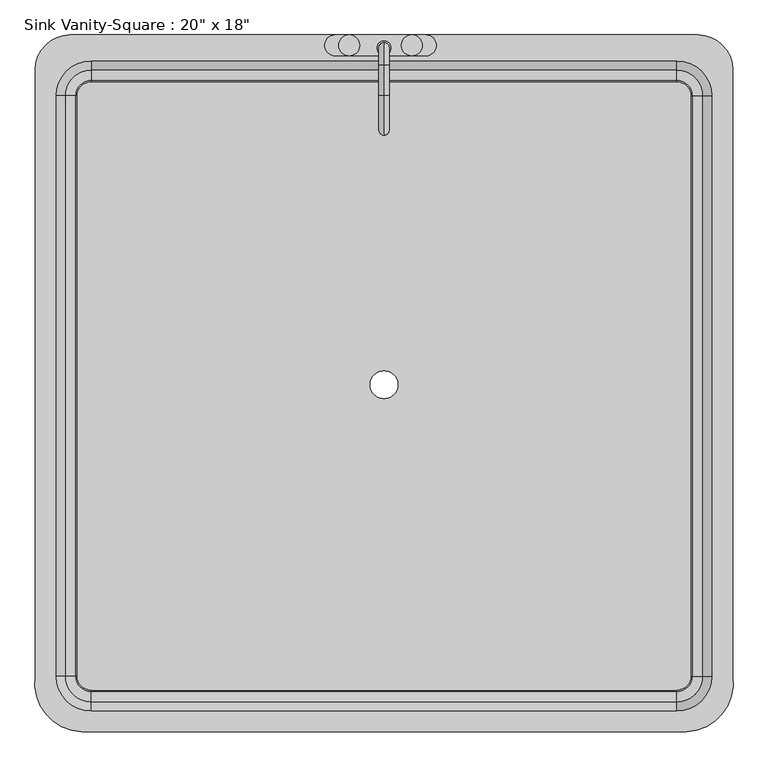
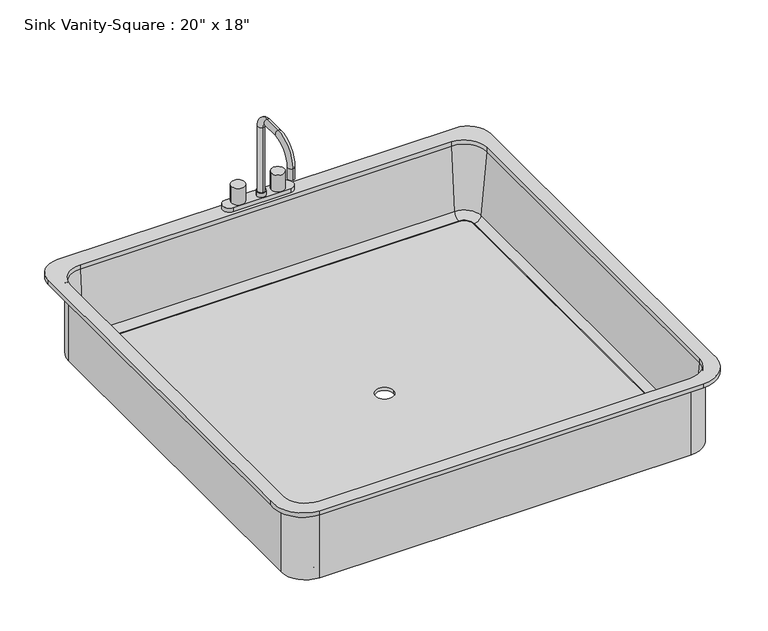
"""IFC4 building model written with IfcOpenShell, lengths in millimetres: flow terminal geometry."""

from ifc_helpers import new_model, si_unit, point, frame, frame_2d, origin, place, context, project, spatial, polyline, circle_curve, ellipse_curve, trimmed, segment, composite_curve, outline, extrude, source, transform, mapped, element, save
from ifc_brep_helpers import plane_surface, cylinder_surface, revolved_surface, advanced_brep


def flow_terminal_6a24c7e0(model_context):
    return source(origin(), model_context, "Body", "SolidModel", [
        extrude(outline(composite_curve([segment(trimmed(circle_curve(frame_2d((549.0892406, 475.4204011)), 25.4), [point((549.0892406, 500.8204011))], [point((574.4892406, 475.4204011))], False, "CARTESIAN"), True, "CONTINUOUS"), segment(polyline([(574.4892406, 475.4204011), (574.4892406, -581.8545989)]), True, "CONTINUOUS"), segment(trimmed(circle_curve(frame_2d((549.0892406, -581.8545989)), 25.4), [point((574.4892406, -581.8545989))], [point((549.0892406, -607.2545989))], False, "CARTESIAN"), True, "CONTINUOUS"), segment(polyline([(549.0892406, -607.2545989), (-517.7107594, -607.2545989)]), True, "CONTINUOUS"), segment(trimmed(circle_curve(frame_2d((-517.7107594, -581.8545989)), 25.4), [point((-517.7107594, -607.2545989))], [point((-543.1107594, -581.8545989))], False, "CARTESIAN"), True, "CONTINUOUS"), segment(polyline([(-543.1107594, -581.8545989), (-543.1107594, 475.4204011)]), True, "CONTINUOUS"), segment(trimmed(circle_curve(frame_2d((-517.7107594, 475.4204011)), 25.4), [point((-543.1107594, 475.4204011))], [point((-517.7107594, 500.8204011))], False, "CARTESIAN"), True, "CONTINUOUS"), segment(polyline([(-517.7107594, 500.8204011), (549.0892406, 500.8204011)]), True, "CONTINUOUS")], self_intersect=False), holes=[composite_curve([segment(trimmed(circle_curve(frame_2d((15.6892406, -50.8)), 25.4), [point((-9.7107594, -50.8))], [point((41.0892406, -50.8))], True, "CARTESIAN"), True, "CONTINUOUS"), segment(trimmed(circle_curve(frame_2d((15.6892406, -50.8)), 25.4), [point((41.0892406, -50.8))], [point((-9.7107594, -50.8))], True, "CARTESIAN"), True, "CONTINUOUS")], self_intersect=False)]), frame((0.0, 0.0, 571.5), z_axis=(0.0, 0.0, 1.0), x_axis=(1.0, 0.0, 0.0)), (0.0, 0.0, 1.0), 9.525),
        extrude(outline(composite_curve([segment(trimmed(circle_curve(frame_2d((-47.8107594, 567.4954011)), 19.05), [point((-66.8607594, 567.4954011))], [point((-28.7607594, 567.4954011))], False, "CARTESIAN"), True, "CONTINUOUS"), segment(trimmed(circle_curve(frame_2d((-47.8107594, 567.4954011)), 19.05), [point((-28.7607594, 567.4954011))], [point((-66.8607594, 567.4954011))], False, "CARTESIAN"), True, "CONTINUOUS")], self_intersect=False)), frame((0.0, 0.0, 812.8), z_axis=(0.0, 0.0, 1.0), x_axis=(1.0, 0.0, 0.0)), (0.0, 0.0, 1.0), 50.8),
        extrude(outline(composite_curve([segment(trimmed(circle_curve(frame_2d((66.4892406, 567.4954011)), 19.05), [point((47.4392406, 567.4954011))], [point((85.5392406, 567.4954011))], False, "CARTESIAN"), True, "CONTINUOUS"), segment(trimmed(circle_curve(frame_2d((66.4892406, 567.4954011)), 19.05), [point((85.5392406, 567.4954011))], [point((47.4392406, 567.4954011))], False, "CARTESIAN"), True, "CONTINUOUS")], self_intersect=False)), frame((0.0, 0.0, 812.8), z_axis=(0.0, 0.0, 1.0), x_axis=(1.0, 0.0, 0.0)), (0.0, 0.0, 1.0), 50.8),
        advanced_brep(
        [(91.8892406, 586.5454011, 800.1), (91.8892406, 548.4454011, 800.1), (-73.2107594, 548.4454011, 800.1), (-73.2107594, 586.5454011, 800.1), (15.6892406, 572.2579011, 1020.7625), (15.6892406, 553.2079011, 1020.7625), (15.6892406, 553.2079011, 825.5), (15.6892406, 572.2579011, 825.5), (15.6892406, 532.5704011, 1060.45), (15.6892406, 532.5704011, 1041.4), (15.6892406, 477.0079011, 1060.45), (15.6892406, 477.0079011, 1041.4), (15.6892406, 403.9829011, 987.425), (15.6892406, 423.0329011, 987.425), (15.6892406, 403.9829011, 952.5), (15.6892406, 423.0329011, 952.5), (2.9892406, 562.7329011, 825.5), (28.3892406, 562.7329011, 825.5), (2.9892406, 562.7329011, 812.8), (28.3892406, 562.7329011, 812.8), (91.8892406, 586.5454011, 812.8), (-73.2107594, 586.5454011, 812.8), (-73.2107594, 548.4454011, 812.8), (91.8892406, 548.4454011, 812.8)],
        [
            (0, 1, circle_curve(frame((91.8892406, 567.4954011, 800.1), z_axis=(0.0, 0.0, -1.0), x_axis=(1.0, 0.0, 0.0)), 19.05)),
            (1, 2),
            (2, 3, circle_curve(frame((-73.2107594, 567.4954011, 800.1), z_axis=(0.0, 0.0, -1.0), x_axis=(1.0, 0.0, 0.0)), 19.05)),
            (3, 0),
            (4, 5, circle_curve(frame((15.6892406, 562.7329011, 1020.7625), z_axis=(0.0, 0.0, -1.0), x_axis=(0.0, -1.0, 0.0)), 9.525)),
            (5, 6),
            (6, 7, circle_curve(frame((15.6892406, 562.7329011, 825.5), z_axis=(0.0, 0.0, 1.0), x_axis=(0.0, -1.0, 0.0)), 9.525)),
            (7, 4),
            (5, 4, circle_curve(frame((15.6892406, 562.7329011, 1020.7625), z_axis=(0.0, 0.0, -1.0), x_axis=(0.0, -1.0, 0.0)), 9.525)),
            (7, 6, circle_curve(frame((15.6892406, 562.7329011, 825.5), z_axis=(0.0, 0.0, 1.0), x_axis=(0.0, -1.0, 0.0)), 9.525)),
            (4, 8, circle_curve(frame((15.6892406, 532.5704011, 1020.7625), z_axis=(1.0, 0.0, 0.0), x_axis=(0.0, 1.0, 0.0)), 39.6875)),
            (8, 9, circle_curve(frame((15.6892406, 532.5704011, 1050.925), z_axis=(0.0, 1.0, 0.0), x_axis=(0.0, 0.0, -1.0)), 9.525)),
            (9, 5, circle_curve(frame((15.6892406, 532.5704011, 1020.7625), z_axis=(-1.0, 0.0, 0.0), x_axis=(0.0, 1.0, 0.0)), 20.6375)),
            (9, 8, circle_curve(frame((15.6892406, 532.5704011, 1050.925), z_axis=(0.0, 1.0, 0.0), x_axis=(0.0, 0.0, -1.0)), 9.525)),
            (8, 10),
            (10, 11, circle_curve(frame((15.6892406, 477.0079011, 1050.925), z_axis=(0.0, 1.0, 0.0), x_axis=(0.0, 0.0, -1.0)), 9.525)),
            (11, 9),
            (11, 10, circle_curve(frame((15.6892406, 477.0079011, 1050.925), z_axis=(0.0, 1.0, 0.0), x_axis=(0.0, 0.0, -1.0)), 9.525)),
            (10, 12, circle_curve(frame((15.6892406, 477.0079011, 987.425), z_axis=(1.0, 0.0, 0.0), x_axis=(0.0, 0.0, 1.0)), 73.025)),
            (12, 13, circle_curve(frame((15.6892406, 413.5079011, 987.425), z_axis=(0.0, 0.0, 1.0), x_axis=(0.0, 1.0, 0.0)), 9.525)),
            (13, 11, circle_curve(frame((15.6892406, 477.0079011, 987.425), z_axis=(-1.0, 0.0, 0.0), x_axis=(0.0, 0.0, 1.0)), 53.975)),
            (13, 12, circle_curve(frame((15.6892406, 413.5079011, 987.425), z_axis=(0.0, 0.0, 1.0), x_axis=(0.0, 1.0, 0.0)), 9.525)),
            (14, 15, circle_curve(frame((15.6892406, 413.5079011, 952.5), z_axis=(0.0, 0.0, -1.0), x_axis=(0.0, 1.0, 0.0)), 9.525)),
            (15, 14, circle_curve(frame((15.6892406, 413.5079011, 952.5), z_axis=(0.0, 0.0, -1.0), x_axis=(0.0, 1.0, 0.0)), 9.525)),
            (12, 14),
            (15, 13),
            (16, 17, circle_curve(frame((15.6892406, 562.7329011, 825.5), z_axis=(0.0, 0.0, 1.0), x_axis=(1.0, 0.0, 0.0)), 12.7)),
            (17, 16, circle_curve(frame((15.6892406, 562.7329011, 825.5), z_axis=(0.0, 0.0, 1.0), x_axis=(1.0, 0.0, 0.0)), 12.7)),
            (16, 18),
            (18, 19, circle_curve(frame((15.6892406, 562.7329011, 812.8), z_axis=(0.0, 0.0, 1.0), x_axis=(1.0, 0.0, 0.0)), 12.7)),
            (19, 17),
            (19, 18, circle_curve(frame((15.6892406, 562.7329011, 812.8), z_axis=(0.0, 0.0, 1.0), x_axis=(1.0, 0.0, 0.0)), 12.7)),
            (20, 21),
            (21, 22, circle_curve(frame((-73.2107594, 567.4954011, 812.8), z_axis=(0.0, 0.0, 1.0), x_axis=(1.0, 0.0, 0.0)), 19.05)),
            (22, 23),
            (23, 20, circle_curve(frame((91.8892406, 567.4954011, 812.8), z_axis=(0.0, 0.0, 1.0), x_axis=(1.0, 0.0, 0.0)), 19.05)),
            (20, 0),
            (3, 21),
            (2, 22),
            (1, 23),
        ],
        [
            plane_surface(frame((15.6892406, 553.2079011, 800.1), z_axis=(0.0, 0.0, -1.0), x_axis=(1.0, 0.0, 0.0))),
            cylinder_surface(frame((15.6892406, 562.7329011, 800.1), z_axis=(0.0, 0.0, -1.0), x_axis=(0.0, -1.0, 0.0)), 9.525),
            revolved_surface(trimmed(ellipse_curve(frame((15.6892406, 562.7329011, 1020.7625), z_axis=(0.0, 0.0, -1.0), x_axis=(0.0, -1.0, 0.0)), 9.525, 9.525), [point((15.6892406, 572.2579011, 1020.7625))], [point((15.6892406, 553.2079011, 1020.7625))], True, "CARTESIAN"), (15.6892406, 532.5704011, 1020.7625), (1.0, 0.0, 0.0)),
            revolved_surface(trimmed(ellipse_curve(frame((15.6892406, 562.7329011, 1020.7625), z_axis=(0.0, 0.0, -1.0), x_axis=(0.0, -1.0, 0.0)), 9.525, 9.525), [point((15.6892406, 553.2079011, 1020.7625))], [point((15.6892406, 572.2579011, 1020.7625))], True, "CARTESIAN"), (15.6892406, 532.5704011, 1020.7625), (1.0, 0.0, 0.0)),
            cylinder_surface(frame((15.6892406, 532.5704011, 1050.925), z_axis=(0.0, 1.0, 0.0), x_axis=(0.0, 0.0, -1.0)), 9.525),
            revolved_surface(trimmed(ellipse_curve(frame((15.6892406, 477.0079011, 1050.925), z_axis=(0.0, 1.0, 0.0), x_axis=(0.0, 0.0, -1.0)), 9.525, 9.525), [point((15.6892406, 477.0079011, 1060.45))], [point((15.6892406, 477.0079011, 1041.4))], True, "CARTESIAN"), (15.6892406, 477.0079011, 987.425), (1.0, 0.0, 0.0)),
            revolved_surface(trimmed(ellipse_curve(frame((15.6892406, 477.0079011, 1050.925), z_axis=(0.0, 1.0, 0.0), x_axis=(0.0, 0.0, -1.0)), 9.525, 9.525), [point((15.6892406, 477.0079011, 1041.4))], [point((15.6892406, 477.0079011, 1060.45))], True, "CARTESIAN"), (15.6892406, 477.0079011, 987.425), (1.0, 0.0, 0.0)),
            plane_surface(frame((15.6892406, 403.9829011, 952.5), z_axis=(0.0, 0.0, -1.0), x_axis=(-1.0, 0.0, 0.0))),
            cylinder_surface(frame((15.6892406, 413.5079011, 987.425), z_axis=(0.0, 0.0, 1.0), x_axis=(0.0, 1.0, 0.0)), 9.525),
            plane_surface(frame((28.3892406, 562.7329011, 825.5), z_axis=(0.0, 0.0, 1.0), x_axis=(0.0, 1.0, 0.0))),
            cylinder_surface(frame((15.6892406, 562.7329011, 812.8), z_axis=(0.0, 0.0, 1.0), x_axis=(1.0, 0.0, 0.0)), 12.7),
            plane_surface(frame((-73.2107594, 586.5454011, 812.8), z_axis=(0.0, 0.0, 1.0), x_axis=(-1.0, 0.0, 0.0))),
            plane_surface(frame((91.8892406, 586.5454011, 812.8), z_axis=(0.0, 1.0, 0.0), x_axis=(0.0, 0.0, -1.0))),
            cylinder_surface(frame((-73.2107594, 567.4954011, 800.1), z_axis=(0.0, 0.0, 1.0), x_axis=(1.0, 0.0, 0.0)), 19.05),
            plane_surface(frame((-73.2107594, 548.4454011, 812.8), z_axis=(0.0, -1.0, 0.0), x_axis=(0.0, 0.0, -1.0))),
            cylinder_surface(frame((91.8892406, 567.4954011, 800.1), z_axis=(0.0, 0.0, 1.0), x_axis=(1.0, 0.0, 0.0)), 19.05),
        ],
        [
            (0, [[1, 2, 3, 4]]),
            (1, [[5, 6, 7, 8]]),
            (1, [[9, -8, 10, -6]]),
            (2, [[-5, 11, 12, 13]]),
            (3, [[-9, -13, 14, -11]]),
            (4, [[-12, 15, 16, 17]]),
            (4, [[-14, -17, 18, -15]]),
            (5, [[-16, 19, 20, 21]]),
            (6, [[-18, -21, 22, -19]]),
            (7, [[23, 24]]),
            (8, [[-20, 25, -24, 26]]),
            (8, [[-22, -26, -23, -25]]),
            (9, [[27, 28], [-7, -10]]),
            (10, [[-27, 29, 30, 31]]),
            (10, [[-28, -31, 32, -29]]),
            (11, [[33, 34, 35, 36], [-30, -32]]),
            (12, [[-33, 37, -4, 38]]),
            (13, [[-34, -38, -3, 39]]),
            (14, [[-35, -39, -2, 40]]),
            (15, [[-36, -40, -1, -37]]),
        ],
    ),
        advanced_brep(
        [(-534.9606923, -683.4545989, 800.1), (566.3391735, -683.4545989, 800.1), (650.6892406, -581.8545989, 800.1), (650.6892406, 523.0454011, 800.1), (587.1892406, 586.5454011, 800.1), (-555.8107593, 586.5454011, 800.1), (-619.3107593, 523.0454011, 800.1), (-619.3107593, -581.8545982, 800.1), (549.0892406, 538.9204011, 800.1), (612.5892406, 475.4204011, 800.1), (612.5892406, -581.8545989, 800.1), (549.0892406, -645.3545989, 800.1), (-517.7107594, -645.3545989, 800.1), (-581.2107594, -581.8545989, 800.1), (-581.2107594, 475.4204011, 800.1), (-517.7107594, 538.9204011, 800.1), (-534.9606923, -683.4545989, 787.4), (-619.3107593, -581.8545982, 787.4), (-619.3107593, 523.0454011, 787.4), (-555.8107593, 586.5454011, 787.4), (587.1892406, 586.5454011, 787.4), (650.6892406, 523.0454011, 787.4), (650.6892406, -581.8545989, 787.4), (566.3391735, -683.4545989, 787.4), (618.9392406, 475.4204011, 787.4), (549.0892406, 545.2704011, 787.4), (-517.7107594, 545.2704011, 787.4), (-587.5607594, 475.4204011, 787.4), (-587.5607594, -581.8545989, 787.4), (-517.7107594, -651.7045989, 787.4), (549.0892406, -651.7045989, 787.4), (618.9392406, -581.8545989, 787.4), (549.0892406, 538.9204011, 787.4), (612.5892406, 475.4204011, 787.4), (612.5892406, -581.8545989, 787.4), (549.0892406, -645.3545989, 787.4), (-517.7107594, -645.3545989, 787.4), (-581.2107594, -581.8545989, 787.4), (-581.2107594, 475.4204011, 787.4), (-517.7107594, 538.9204011, 787.4), (618.9392406, 475.4204011, 571.5), (549.0892406, 545.2704011, 571.5), (574.4892406, 475.4204011, 571.5), (549.0892406, 500.8204011, 571.5), (574.4892406, 475.4204011, 581.025), (549.0892406, 500.8204011, 581.025), (577.0776588, 475.4204011, 581.025), (549.0892406, 503.4088193, 581.025), (596.0551678, 475.4204011, 598.4146831), (549.0892406, 522.3863283, 598.4146831), (618.9392406, -581.8545989, 571.5), (574.4892406, -581.8545989, 571.5), (574.4892406, -581.8545989, 581.025), (577.0776588, -581.8545989, 581.025), (596.0551678, -581.8545989, 598.4146831), (549.0892406, -651.7045989, 571.5), (549.0892406, -607.2545989, 571.5), (549.0892406, -607.2545989, 581.025), (549.0892406, -609.8430171, 581.025), (549.0892406, -628.8205261, 598.4146831), (-517.7107594, -651.7045989, 571.5), (-517.7107594, -607.2545989, 571.5), (-517.7107594, -607.2545989, 581.025), (-517.7107594, -609.8430171, 581.025), (-517.7107594, -628.8205261, 598.4146831), (-587.5607594, -581.8545989, 571.5), (-543.1107594, -581.8545989, 571.5), (-543.1107594, -581.8545989, 581.025), (-545.6991776, -581.8545989, 581.025), (-564.6766866, -581.8545989, 598.4146831), (-587.5607594, 475.4204011, 571.5), (-543.1107594, 475.4204011, 571.5), (-543.1107594, 475.4204011, 581.025), (-545.6991776, 475.4204011, 581.025), (-564.6766866, 475.4204011, 598.4146831), (-517.7107594, 545.2704011, 571.5), (-517.7107594, 500.8204011, 571.5), (-517.7107594, 500.8204011, 581.025), (-517.7107594, 503.4088193, 581.025), (-517.7107594, 522.3863283, 598.4146831)],
        [
            (0, 1),
            (1, 2, circle_curve(frame((562.5319557, -594.4793432, 800.1), z_axis=(0.0, 0.0, 1.0), x_axis=(1.0, 0.0, 0.0)), 89.0566732)),
            (2, 3),
            (3, 4, circle_curve(frame((587.1892406, 523.0454011, 800.1), z_axis=(0.0, 0.0, 1.0), x_axis=(1.0, 0.0, 0.0)), 63.5)),
            (4, 5),
            (5, 6, circle_curve(frame((-555.8107593, 523.0454011, 800.1), z_axis=(0.0, 0.0, 1.0), x_axis=(1.0, 0.0, 0.0)), 63.5)),
            (6, 7),
            (7, 0, circle_curve(frame((-531.1534746, -594.4793432, 800.1), z_axis=(0.0, 0.0, 1.0), x_axis=(1.0, 0.0, 0.0)), 89.0566732)),
            (8, 9, circle_curve(frame((549.0892406, 475.4204011, 800.1), z_axis=(0.0, 0.0, -1.0), x_axis=(1.0, 0.0, 0.0)), 63.5)),
            (9, 10),
            (10, 11, circle_curve(frame((549.0892406, -581.8545989, 800.1), z_axis=(0.0, 0.0, -1.0), x_axis=(1.0, 0.0, 0.0)), 63.5)),
            (11, 12),
            (12, 13, circle_curve(frame((-517.7107594, -581.8545989, 800.1), z_axis=(0.0, 0.0, -1.0), x_axis=(1.0, 0.0, 0.0)), 63.5)),
            (13, 14),
            (14, 15, circle_curve(frame((-517.7107594, 475.4204011, 800.1), z_axis=(0.0, 0.0, -1.0), x_axis=(1.0, 0.0, 0.0)), 63.5)),
            (15, 8),
            (16, 17, circle_curve(frame((-531.1534746, -594.4793432, 787.4), z_axis=(0.0, 0.0, -1.0), x_axis=(1.0, 0.0, 0.0)), 89.0566732)),
            (17, 18),
            (18, 19, circle_curve(frame((-555.8107593, 523.0454011, 787.4), z_axis=(0.0, 0.0, -1.0), x_axis=(1.0, 0.0, 0.0)), 63.5)),
            (19, 20),
            (20, 21, circle_curve(frame((587.1892406, 523.0454011, 787.4), z_axis=(0.0, 0.0, -1.0), x_axis=(1.0, 0.0, 0.0)), 63.5)),
            (21, 22),
            (22, 23, circle_curve(frame((562.5319557, -594.4793432, 787.4), z_axis=(0.0, 0.0, -1.0), x_axis=(1.0, 0.0, 0.0)), 89.0566732)),
            (23, 16),
            (24, 25, circle_curve(frame((549.0892406, 475.4204011, 787.4), z_axis=(0.0, 0.0, 1.0), x_axis=(0.0, 1.0, 0.0)), 69.85)),
            (25, 26),
            (26, 27, circle_curve(frame((-517.7107594, 475.4204011, 787.4), z_axis=(0.0, 0.0, 1.0), x_axis=(-1.0, 0.0, 0.0)), 69.85)),
            (27, 28),
            (28, 29, circle_curve(frame((-517.7107594, -581.8545989, 787.4), z_axis=(0.0, 0.0, 1.0), x_axis=(0.0, -1.0, 0.0)), 69.85)),
            (29, 30),
            (30, 31, circle_curve(frame((549.0892406, -581.8545989, 787.4), z_axis=(0.0, 0.0, 1.0), x_axis=(1.0, 0.0, 0.0)), 69.85)),
            (31, 24),
            (0, 16),
            (23, 1),
            (22, 2),
            (21, 3),
            (20, 4),
            (19, 5),
            (18, 6),
            (17, 7),
            (8, 32),
            (32, 33, circle_curve(frame((549.0892406, 475.4204011, 787.4), z_axis=(0.0, 0.0, -1.0), x_axis=(1.0, 0.0, 0.0)), 63.5)),
            (33, 9),
            (33, 34),
            (34, 10),
            (34, 35, circle_curve(frame((549.0892406, -581.8545989, 787.4), z_axis=(0.0, 0.0, -1.0), x_axis=(1.0, 0.0, 0.0)), 63.5)),
            (35, 11),
            (35, 36),
            (36, 12),
            (36, 37, circle_curve(frame((-517.7107594, -581.8545989, 787.4), z_axis=(0.0, 0.0, -1.0), x_axis=(1.0, 0.0, 0.0)), 63.5)),
            (37, 13),
            (37, 38),
            (38, 14),
            (38, 39, circle_curve(frame((-517.7107594, 475.4204011, 787.4), z_axis=(0.0, 0.0, -1.0), x_axis=(1.0, 0.0, 0.0)), 63.5)),
            (39, 15),
            (39, 32),
            (40, 41, circle_curve(frame((549.0892406, 475.4204011, 571.5), z_axis=(0.0, 0.0, 1.0), x_axis=(0.0, 1.0, 0.0)), 69.85)),
            (41, 25),
            (24, 40),
            (40, 42),
            (42, 43, circle_curve(frame((549.0892406, 475.4204011, 571.5), z_axis=(0.0, 0.0, 1.0), x_axis=(0.0, 1.0, 0.0)), 25.4)),
            (43, 41),
            (42, 44),
            (44, 45, circle_curve(frame((549.0892406, 475.4204011, 581.025), z_axis=(0.0, 0.0, 1.0), x_axis=(0.0, 1.0, 0.0)), 25.4)),
            (45, 43),
            (44, 46),
            (46, 47, circle_curve(frame((549.0892406, 475.4204011, 581.025), z_axis=(0.0, 0.0, 1.0), x_axis=(0.0, 1.0, 0.0)), 27.9884182)),
            (47, 45),
            (46, 48, circle_curve(frame((577.0776588, 475.4204011, 600.075), z_axis=(0.0, -1.0, 0.0), x_axis=(1.0, 0.0, 0.0)), 19.05)),
            (48, 49, circle_curve(frame((549.0892406, 475.4204011, 598.4146831), z_axis=(0.0, 0.0, 1.0), x_axis=(0.0, 1.0, 0.0)), 46.9659272)),
            (49, 47, circle_curve(frame((549.0892406, 503.4088193, 600.075), z_axis=(-1.0, 0.0, 0.0), x_axis=(0.0, 1.0, 0.0)), 19.05)),
            (48, 33),
            (32, 49),
            (31, 50),
            (50, 40),
            (50, 51),
            (51, 42),
            (51, 52),
            (52, 44),
            (52, 53),
            (53, 46),
            (53, 54, circle_curve(frame((577.0776588, -581.8545989, 600.075), z_axis=(0.0, -1.0, 0.0), x_axis=(1.0, 0.0, 0.0)), 19.05)),
            (54, 48),
            (54, 34),
            (30, 55),
            (55, 50, circle_curve(frame((549.0892406, -581.8545989, 571.5), z_axis=(0.0, 0.0, 1.0), x_axis=(1.0, 0.0, 0.0)), 69.85)),
            (55, 56),
            (56, 51, circle_curve(frame((549.0892406, -581.8545989, 571.5), z_axis=(0.0, 0.0, 1.0), x_axis=(1.0, 0.0, 0.0)), 25.4)),
            (56, 57),
            (57, 52, circle_curve(frame((549.0892406, -581.8545989, 581.025), z_axis=(0.0, 0.0, 1.0), x_axis=(1.0, 0.0, 0.0)), 25.4)),
            (57, 58),
            (58, 53, circle_curve(frame((549.0892406, -581.8545989, 581.025), z_axis=(0.0, 0.0, 1.0), x_axis=(1.0, 0.0, 0.0)), 27.9884182)),
            (58, 59, circle_curve(frame((549.0892406, -609.8430171, 600.075), z_axis=(-1.0, 0.0, 0.0), x_axis=(0.0, -1.0, 0.0)), 19.05)),
            (59, 54, circle_curve(frame((549.0892406, -581.8545989, 598.4146831), z_axis=(0.0, 0.0, 1.0), x_axis=(1.0, 0.0, 0.0)), 46.9659272)),
            (59, 35),
            (29, 60),
            (60, 55),
            (60, 61),
            (61, 56),
            (61, 62),
            (62, 57),
            (62, 63),
            (63, 58),
            (63, 64, circle_curve(frame((-517.7107594, -609.8430171, 600.075), z_axis=(-1.0, 0.0, 0.0), x_axis=(0.0, -1.0, 0.0)), 19.05)),
            (64, 59),
            (64, 36),
            (28, 65),
            (65, 60, circle_curve(frame((-517.7107594, -581.8545989, 571.5), z_axis=(0.0, 0.0, 1.0), x_axis=(0.0, -1.0, 0.0)), 69.85)),
            (65, 66),
            (66, 61, circle_curve(frame((-517.7107594, -581.8545989, 571.5), z_axis=(0.0, 0.0, 1.0), x_axis=(0.0, -1.0, 0.0)), 25.4)),
            (66, 67),
            (67, 62, circle_curve(frame((-517.7107594, -581.8545989, 581.025), z_axis=(0.0, 0.0, 1.0), x_axis=(0.0, -1.0, 0.0)), 25.4)),
            (67, 68),
            (68, 63, circle_curve(frame((-517.7107594, -581.8545989, 581.025), z_axis=(0.0, 0.0, 1.0), x_axis=(0.0, -1.0, 0.0)), 27.9884182)),
            (68, 69, circle_curve(frame((-545.6991776, -581.8545989, 600.075), z_axis=(0.0, 1.0, 0.0), x_axis=(-1.0, 0.0, 0.0)), 19.05)),
            (69, 64, circle_curve(frame((-517.7107594, -581.8545989, 598.4146831), z_axis=(0.0, 0.0, 1.0), x_axis=(0.0, -1.0, 0.0)), 46.9659272)),
            (69, 37),
            (27, 70),
            (70, 65),
            (70, 71),
            (71, 66),
            (71, 72),
            (72, 67),
            (72, 73),
            (73, 68),
            (73, 74, circle_curve(frame((-545.6991776, 475.4204011, 600.075), z_axis=(0.0, 1.0, 0.0), x_axis=(-1.0, 0.0, 0.0)), 19.05)),
            (74, 69),
            (74, 38),
            (26, 75),
            (75, 70, circle_curve(frame((-517.7107594, 475.4204011, 571.5), z_axis=(0.0, 0.0, 1.0), x_axis=(-1.0, 0.0, 0.0)), 69.85)),
            (75, 76),
            (76, 71, circle_curve(frame((-517.7107594, 475.4204011, 571.5), z_axis=(0.0, 0.0, 1.0), x_axis=(-1.0, 0.0, 0.0)), 25.4)),
            (76, 77),
            (77, 72, circle_curve(frame((-517.7107594, 475.4204011, 581.025), z_axis=(0.0, 0.0, 1.0), x_axis=(-1.0, 0.0, 0.0)), 25.4)),
            (77, 78),
            (78, 73, circle_curve(frame((-517.7107594, 475.4204011, 581.025), z_axis=(0.0, 0.0, 1.0), x_axis=(-1.0, 0.0, 0.0)), 27.9884182)),
            (78, 79, circle_curve(frame((-517.7107594, 503.4088193, 600.075), z_axis=(1.0, 0.0, 0.0), x_axis=(0.0, 1.0, 0.0)), 19.05)),
            (79, 74, circle_curve(frame((-517.7107594, 475.4204011, 598.4146831), z_axis=(0.0, 0.0, 1.0), x_axis=(-1.0, 0.0, 0.0)), 46.9659272)),
            (79, 39),
            (41, 75),
            (43, 76),
            (45, 77),
            (47, 78),
            (49, 79),
        ],
        [
            plane_surface(frame((566.3391735, -683.4545989, 800.1), z_axis=(0.0, 0.0, 1.0), x_axis=(1.0, 0.0, 0.0))),
            plane_surface(frame((566.3391735, -683.4545989, 787.4), z_axis=(0.0, 0.0, -1.0), x_axis=(-1.0, 0.0, 0.0))),
            plane_surface(frame((-534.9606923, -683.4545989, 800.1), z_axis=(0.0, -1.0, 0.0), x_axis=(0.0, 0.0, -1.0))),
            cylinder_surface(frame((562.5319557, -594.4793432, 787.4), z_axis=(0.0, 0.0, 1.0), x_axis=(1.0, 0.0, 0.0)), 89.0566732),
            plane_surface(frame((650.6892406, -581.8545989, 800.1), z_axis=(1.0, 0.0, 0.0), x_axis=(0.0, 0.0, -1.0))),
            cylinder_surface(frame((587.1892406, 523.0454011, 787.4), z_axis=(0.0, 0.0, 1.0), x_axis=(1.0, 0.0, 0.0)), 63.5),
            plane_surface(frame((587.1892406, 586.5454011, 800.1), z_axis=(0.0, 1.0, 0.0), x_axis=(0.0, 0.0, -1.0))),
            cylinder_surface(frame((-555.8107593, 523.0454011, 787.4), z_axis=(0.0, 0.0, 1.0), x_axis=(1.0, 0.0, 0.0)), 63.5),
            plane_surface(frame((-619.3107593, 523.0454011, 800.1), z_axis=(-1.0, 0.0, 0.0), x_axis=(0.0, 0.0, -1.0))),
            cylinder_surface(frame((-531.1534746, -594.4793432, 787.4), z_axis=(0.0, 0.0, 1.0), x_axis=(1.0, 0.0, 0.0)), 89.0566732),
            revolved_surface(polyline([(612.5892406, 475.4204011, 787.4), (612.5892406, 475.4204011, 800.1)]), (549.0892406, 475.4204011, 0.0), (0.0, 0.0, -1.0)),
            plane_surface(frame((612.5892406, 475.4204011, 800.1), z_axis=(-1.0, 0.0, 0.0), x_axis=(0.0, 0.0, -1.0))),
            revolved_surface(polyline([(612.5892406, -581.8545989, 787.4), (612.5892406, -581.8545989, 800.1)]), (549.0892406, -581.8545989, 0.0), (0.0, 0.0, -1.0)),
            plane_surface(frame((549.0892406, -645.3545989, 800.1), z_axis=(0.0, 1.0, 0.0), x_axis=(0.0, 0.0, -1.0))),
            revolved_surface(polyline([(-454.21075940000003, -581.8545989, 787.4), (-454.21075940000003, -581.8545989, 800.1)]), (-517.7107594, -581.8545989, 0.0), (0.0, 0.0, -1.0)),
            plane_surface(frame((-581.2107594, -581.8545989, 800.1), z_axis=(1.0, 0.0, 0.0), x_axis=(0.0, 0.0, -1.0))),
            revolved_surface(polyline([(-454.21075940000003, 475.4204011, 787.4), (-454.21075940000003, 475.4204011, 800.1)]), (-517.7107594, 475.4204011, 0.0), (0.0, 0.0, -1.0)),
            plane_surface(frame((-517.7107594, 538.9204011, 800.1), z_axis=(0.0, -1.0, 0.0), x_axis=(0.0, 0.0, -1.0))),
            cylinder_surface(frame((549.0892406, 475.4204011, 0.0), z_axis=(0.0, 0.0, -1.0), x_axis=(0.0, 1.0, 0.0)), 69.85),
            plane_surface(frame((549.0892406, 475.4204011, 571.5), z_axis=(0.0, 0.0, -1.0), x_axis=(0.0, 1.0, 0.0))),
            revolved_surface(polyline([(549.0892406, 500.82040109999997, 571.5), (549.0892406, 500.82040109999997, 581.025)]), (549.0892406, 475.4204011, 0.0), (0.0, 0.0, -1.0)),
            plane_surface(frame((549.0892406, 475.4204011, 581.025), z_axis=(0.0, 0.0, 1.0), x_axis=(0.0, 1.0, 0.0))),
            revolved_surface(trimmed(ellipse_curve(frame((549.0892406, 503.4088193, 600.075), z_axis=(1.0, 0.0, 0.0), x_axis=(0.0, 1.0, 0.0)), 19.05, 19.05), [point((549.0892406, 503.4088193, 581.025))], [point((549.0892406, 522.3863283, 598.4146831))], True, "CARTESIAN"), (549.0892406, 475.4204011, 0.0), (0.0, 0.0, -1.0)),
            revolved_surface(polyline([(549.0892406, 522.3863283, 598.4146831), (549.0892406, 538.9204011, 787.4)]), (549.0892406, 475.4204011, 0.0), (0.0, 0.0, -1.0)),
            plane_surface(frame((618.9392406, 475.4204011, 787.4), z_axis=(1.0, 0.0, 0.0), x_axis=(0.0, -1.0, 0.0))),
            plane_surface(frame((618.9392406, 475.4204011, 571.5), z_axis=(0.0, 0.0, -1.0), x_axis=(0.0, -1.0, 0.0))),
            plane_surface(frame((574.4892406, 475.4204011, 571.5), z_axis=(-1.0, 0.0, 0.0), x_axis=(0.0, -1.0, 0.0))),
            plane_surface(frame((574.4892406, 475.4204011, 581.025), z_axis=(0.0, 0.0, 1.0), x_axis=(0.0, -1.0, 0.0))),
            revolved_surface(polyline([(596.1276588, -581.8545989000002, 600.075), (596.1276588, 475.4204011, 600.075)]), (577.0776588, 475.4204011, 600.075), (0.0, -1.0, 0.0)),
            plane_surface(frame((596.0551678, 475.4204011, 598.4146831), z_axis=(-0.9961946980917442, 0.0, 0.08715574274767408), x_axis=(0.0, -1.0, 0.0))),
            cylinder_surface(frame((549.0892406, -581.8545989, 0.0), z_axis=(0.0, 0.0, -1.0), x_axis=(1.0, 0.0, 0.0)), 69.85),
            plane_surface(frame((549.0892406, -581.8545989, 571.5), z_axis=(0.0, 0.0, -1.0), x_axis=(1.0, 0.0, 0.0))),
            revolved_surface(polyline([(574.4892406, -581.8545989, 571.5), (574.4892406, -581.8545989, 581.025)]), (549.0892406, -581.8545989, 0.0), (0.0, 0.0, -1.0)),
            plane_surface(frame((549.0892406, -581.8545989, 581.025), z_axis=(0.0, 0.0, 1.0), x_axis=(1.0, 0.0, 0.0))),
            revolved_surface(trimmed(ellipse_curve(frame((577.0776588, -581.8545989, 600.075), z_axis=(0.0, -1.0, 0.0), x_axis=(1.0, 0.0, 0.0)), 19.05, 19.05), [point((577.0776588, -581.8545989, 581.025))], [point((596.0551678, -581.8545989, 598.4146831))], True, "CARTESIAN"), (549.0892406, -581.8545989, 0.0), (0.0, 0.0, -1.0)),
            revolved_surface(polyline([(596.0551678, -581.8545989, 598.4146831), (612.5892406, -581.8545989, 787.4)]), (549.0892406, -581.8545989, 0.0), (0.0, 0.0, -1.0)),
            plane_surface(frame((549.0892406, -651.7045989, 787.4), z_axis=(0.0, -1.0, 0.0), x_axis=(-1.0, 0.0, 0.0))),
            plane_surface(frame((549.0892406, -651.7045989, 571.5), z_axis=(0.0, 0.0, -1.0), x_axis=(-1.0, 0.0, 0.0))),
            plane_surface(frame((549.0892406, -607.2545989, 571.5), z_axis=(0.0, 1.0, 0.0), x_axis=(-1.0, 0.0, 0.0))),
            plane_surface(frame((549.0892406, -607.2545989, 581.025), z_axis=(0.0, 0.0, 1.0), x_axis=(-1.0, 0.0, 0.0))),
            revolved_surface(polyline([(-517.7107594000001, -628.8930171, 600.075), (549.0892406, -628.8930171, 600.075)]), (549.0892406, -609.8430171, 600.075), (-1.0, 0.0, 0.0)),
            plane_surface(frame((549.0892406, -628.8205261, 598.4146831), z_axis=(0.0, 0.9961946980917442, 0.08715574274767408), x_axis=(-1.0, 0.0, 0.0))),
            cylinder_surface(frame((-517.7107594, -581.8545989, 0.0), z_axis=(0.0, 0.0, -1.0), x_axis=(0.0, -1.0, 0.0)), 69.85),
            plane_surface(frame((-517.7107594, -581.8545989, 571.5), z_axis=(0.0, 0.0, -1.0), x_axis=(0.0, -1.0, 0.0))),
            revolved_surface(polyline([(-517.7107594, -607.2545989, 571.5), (-517.7107594, -607.2545989, 581.025)]), (-517.7107594, -581.8545989, 0.0), (0.0, 0.0, -1.0)),
            plane_surface(frame((-517.7107594, -581.8545989, 581.025), z_axis=(0.0, 0.0, 1.0), x_axis=(0.0, -1.0, 0.0))),
            revolved_surface(trimmed(ellipse_curve(frame((-517.7107594, -609.8430171, 600.075), z_axis=(-1.0, 0.0, 0.0), x_axis=(0.0, -1.0, 0.0)), 19.05, 19.05), [point((-517.7107594, -609.8430171, 581.025))], [point((-517.7107594, -628.8205261, 598.4146831))], True, "CARTESIAN"), (-517.7107594, -581.8545989, 0.0), (0.0, 0.0, -1.0)),
            revolved_surface(polyline([(-517.7107594, -628.8205261, 598.4146831), (-517.7107594, -645.3545989, 787.4)]), (-517.7107594, -581.8545989, 0.0), (0.0, 0.0, -1.0)),
            plane_surface(frame((-587.5607594, -581.8545989, 787.4), z_axis=(-1.0, 0.0, 0.0), x_axis=(0.0, 1.0, 0.0))),
            plane_surface(frame((-587.5607594, -581.8545989, 571.5), z_axis=(0.0, 0.0, -1.0), x_axis=(0.0, 1.0, 0.0))),
            plane_surface(frame((-543.1107594, -581.8545989, 571.5), z_axis=(1.0, 0.0, 0.0), x_axis=(0.0, 1.0, 0.0))),
            plane_surface(frame((-543.1107594, -581.8545989, 581.025), z_axis=(0.0, 0.0, 1.0), x_axis=(0.0, 1.0, 0.0))),
            revolved_surface(polyline([(-564.7491775999999, 475.42040110000005, 600.075), (-564.7491775999999, -581.8545989, 600.075)]), (-545.6991776, -581.8545989, 600.075), (0.0, 1.0, 0.0)),
            plane_surface(frame((-564.6766866, -581.8545989, 598.4146831), z_axis=(0.9961946980917442, 0.0, 0.08715574274767408), x_axis=(0.0, 1.0, 0.0))),
            cylinder_surface(frame((-517.7107594, 475.4204011, 0.0), z_axis=(0.0, 0.0, -1.0), x_axis=(-1.0, 0.0, 0.0)), 69.85),
            plane_surface(frame((-517.7107594, 475.4204011, 571.5), z_axis=(0.0, 0.0, -1.0), x_axis=(-1.0, 0.0, 0.0))),
            revolved_surface(polyline([(-543.1107594, 475.4204011, 571.5), (-543.1107594, 475.4204011, 581.025)]), (-517.7107594, 475.4204011, 0.0), (0.0, 0.0, -1.0)),
            plane_surface(frame((-517.7107594, 475.4204011, 581.025), z_axis=(0.0, 0.0, 1.0), x_axis=(-1.0, 0.0, 0.0))),
            revolved_surface(trimmed(ellipse_curve(frame((-545.6991776, 475.4204011, 600.075), z_axis=(0.0, 1.0, 0.0), x_axis=(-1.0, 0.0, 0.0)), 19.05, 19.05), [point((-545.6991776, 475.4204011, 581.025))], [point((-564.6766866, 475.4204011, 598.4146831))], True, "CARTESIAN"), (-517.7107594, 475.4204011, 0.0), (0.0, 0.0, -1.0)),
            revolved_surface(polyline([(-564.6766866, 475.4204011, 598.4146831), (-581.2107594, 475.4204011, 787.4)]), (-517.7107594, 475.4204011, 0.0), (0.0, 0.0, -1.0)),
            plane_surface(frame((-517.7107594, 545.2704011, 787.4), z_axis=(0.0, 1.0, 0.0), x_axis=(1.0, 0.0, 0.0))),
            plane_surface(frame((-517.7107594, 545.2704011, 571.5), z_axis=(0.0, 0.0, -1.0), x_axis=(1.0, 0.0, 0.0))),
            plane_surface(frame((-517.7107594, 500.8204011, 571.5), z_axis=(0.0, -1.0, 0.0), x_axis=(1.0, 0.0, 0.0))),
            plane_surface(frame((-517.7107594, 500.8204011, 581.025), z_axis=(0.0, 0.0, 1.0), x_axis=(1.0, 0.0, 0.0))),
            revolved_surface(polyline([(549.0892406000002, 522.4588193, 600.075), (-517.7107594, 522.4588193, 600.075)]), (-517.7107594, 503.4088193, 600.075), (1.0, 0.0, 0.0)),
            plane_surface(frame((-517.7107594, 522.3863283, 598.4146831), z_axis=(0.0, -0.9961946980917442, 0.08715574274767408), x_axis=(1.0, 0.0, 0.0))),
        ],
        [
            (0, [[1, 2, 3, 4, 5, 6, 7, 8], [9, 10, 11, 12, 13, 14, 15, 16]]),
            (1, [[17, 18, 19, 20, 21, 22, 23, 24], [25, 26, 27, 28, 29, 30, 31, 32]]),
            (2, [[-1, 33, -24, 34]]),
            (3, [[-2, -34, -23, 35]]),
            (4, [[-3, -35, -22, 36]]),
            (5, [[-4, -36, -21, 37]]),
            (6, [[-5, -37, -20, 38]]),
            (7, [[-6, -38, -19, 39]]),
            (8, [[-7, -39, -18, 40]]),
            (9, [[-8, -40, -17, -33]]),
            (10, [[-9, 41, 42, 43]]),
            (11, [[-10, -43, 44, 45]]),
            (12, [[-11, -45, 46, 47]]),
            (13, [[-12, -47, 48, 49]]),
            (14, [[-13, -49, 50, 51]]),
            (15, [[-14, -51, 52, 53]]),
            (16, [[-15, -53, 54, 55]]),
            (17, [[-16, -55, 56, -41]]),
            (18, [[57, 58, -25, 59]]),
            (19, [[-57, 60, 61, 62]]),
            (20, [[-61, 63, 64, 65]]),
            (21, [[-64, 66, 67, 68]]),
            (22, [[-67, 69, 70, 71]]),
            (23, [[-70, 72, -42, 73]]),
            (24, [[-59, -32, 74, 75]]),
            (25, [[-60, -75, 76, 77]]),
            (26, [[-63, -77, 78, 79]]),
            (27, [[-66, -79, 80, 81]]),
            (28, [[-69, -81, 82, 83]]),
            (29, [[-72, -83, 84, -44]]),
            (30, [[-74, -31, 85, 86]]),
            (31, [[-76, -86, 87, 88]]),
            (32, [[-78, -88, 89, 90]]),
            (33, [[-80, -90, 91, 92]]),
            (34, [[-82, -92, 93, 94]]),
            (35, [[-84, -94, 95, -46]]),
            (36, [[-85, -30, 96, 97]]),
            (37, [[-87, -97, 98, 99]]),
            (38, [[-89, -99, 100, 101]]),
            (39, [[-91, -101, 102, 103]]),
            (40, [[-93, -103, 104, 105]]),
            (41, [[-95, -105, 106, -48]]),
            (42, [[-96, -29, 107, 108]]),
            (43, [[-98, -108, 109, 110]]),
            (44, [[-100, -110, 111, 112]]),
            (45, [[-102, -112, 113, 114]]),
            (46, [[-104, -114, 115, 116]]),
            (47, [[-106, -116, 117, -50]]),
            (48, [[-107, -28, 118, 119]]),
            (49, [[-109, -119, 120, 121]]),
            (50, [[-111, -121, 122, 123]]),
            (51, [[-113, -123, 124, 125]]),
            (52, [[-115, -125, 126, 127]]),
            (53, [[-117, -127, 128, -52]]),
            (54, [[-118, -27, 129, 130]]),
            (55, [[-120, -130, 131, 132]]),
            (56, [[-122, -132, 133, 134]]),
            (57, [[-124, -134, 135, 136]]),
            (58, [[-126, -136, 137, 138]]),
            (59, [[-128, -138, 139, -54]]),
            (60, [[-58, 140, -129, -26]]),
            (61, [[-62, 141, -131, -140]]),
            (62, [[-65, 142, -133, -141]]),
            (63, [[-68, 143, -135, -142]]),
            (64, [[-71, 144, -137, -143]]),
            (65, [[-73, -56, -139, -144]]),
        ],
    ),
    ])


if __name__ == "__main__":
    model = new_model("IFC4")
    model_context = context("Model", 3, world=origin())
    ifc_project = project(units=[si_unit("LENGTHUNIT", "METRE", prefix="MILLI")], contexts=[model_context])
    site = spatial("IfcSite", under=ifc_project)
    building = spatial("IfcBuilding", under=site)
    placement = place(None, origin())
    flow_terminal_shape = flow_terminal_6a24c7e0(model_context)
    element("IfcFlowTerminal", 1, ObjectType="Sink Vanity-Square : 20\" x 18\"", at=placement, inside=building, context=model_context, shape_type="MappedRepresentation", body=[
        mapped(flow_terminal_shape, transform((0.0, 0.0, 0.0), x_axis=(1.0, 0.0, 0.0), y_axis=(0.0, 1.0, 0.0), z_axis=(0.0, 0.0, 1.0))),
    ])
    save(model, "model.ifc")

# Revit data of these elements
# Type "Sink Vanity-Square : 20\" x 18\""
#   Assembly Code = "D2010400"
#   Counter Height = 2' - 7"
#   Depth = 4' - 2"
#   Width = 4' - 2"
#   Basin Material = Porcelain, Linen
#   Faucet Material = Steel, Polished
#   Default Elevation = 0
# Element 1 (IfcFlowTerminal, "Sink Vanity-Square : 20\" x 18\"")
#   Materials on its faces: "Porcelain, Linen", "Steel, Polished"
# Materials
#   "Porcelain, Linen": class "Ceramic", colour RGB 249 239 230, transparency 0, Description = "Porcelain, linen", Cost = 0
#   "Steel, Polished": class "Metal", colour RGB 57 57 57, transparency 0, Description = "Polished steel", Cost = 0
